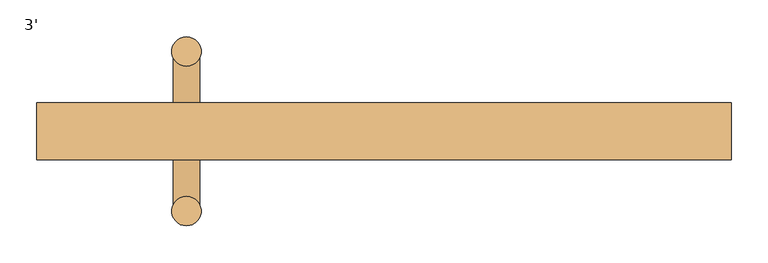
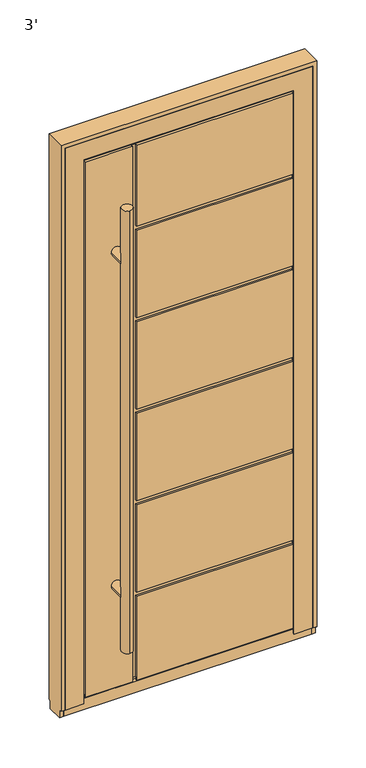
"""IFC4 building model written with IfcOpenShell, lengths in millimetres: door geometry, 3'."""

from ifc_helpers import new_model, si_unit, point, frame, frame_2d, origin, place, context, project, spatial, circle_curve, trimmed, segment, composite_curve, outline, extrude, faceted_brep, source, transform, mapped, element, save


def door_3_5c4206ef(model_context):
    return source(origin(), model_context, "Body", "SolidModel", [
        extrude(outline(composite_curve([segment(trimmed(circle_curve(frame_2d((-268.65, -90.8003001)), 20.0), [point((-268.65, -70.8003001))], [point((-268.65, -110.8003001))], False, "CARTESIAN"), True, "CONTINUOUS"), segment(trimmed(circle_curve(frame_2d((-268.65, -90.8003001)), 20.0), [point((-268.65, -110.8003001))], [point((-268.65, -70.8003001))], False, "CARTESIAN"), True, "CONTINUOUS")], self_intersect=False)), frame((0.0, 0.0, 210.0000003), z_axis=(0.0, 0.0, 1.0), x_axis=(1.0, 0.0, 0.0)), (0.0, 0.0, 1.0), 1724.5),
        extrude(outline(composite_curve([segment(trimmed(circle_curve(frame_2d((-268.65, 126.2003001)), 20.0), [point((-268.65, 146.2003001))], [point((-268.65, 106.2003001))], False, "CARTESIAN"), True, "CONTINUOUS"), segment(trimmed(circle_curve(frame_2d((-268.65, 126.2003001)), 20.0), [point((-268.65, 106.2003001))], [point((-268.65, 146.2003001))], False, "CARTESIAN"), True, "CONTINUOUS")], self_intersect=False)), frame((0.0, 0.0, 210.0000003), z_axis=(0.0, 0.0, 1.0), x_axis=(1.0, 0.0, 0.0)), (0.0, 0.0, 1.0), 1724.5),
        extrude(outline(composite_curve([segment(trimmed(circle_curve(frame_2d((422.2500003, -268.65)), 18.0), [point((422.2500003, -286.65))], [point((422.2500003, -250.65))], False, "CARTESIAN"), True, "CONTINUOUS"), segment(trimmed(circle_curve(frame_2d((422.2500003, -268.65)), 18.0), [point((422.2500003, -250.65))], [point((422.2500003, -286.65))], False, "CARTESIAN"), True, "CONTINUOUS")], self_intersect=False)), frame((0.0, -90.8, 0.0), z_axis=(0.0, 1.0, 0.0), x_axis=(0.0, 0.0, 1.0)), (0.0, 0.0, 1.0), 217.0),
        extrude(outline(composite_curve([segment(trimmed(circle_curve(frame_2d((1722.2500003, -268.65)), 18.0), [point((1722.2500003, -286.65))], [point((1722.2500003, -250.65))], False, "CARTESIAN"), True, "CONTINUOUS"), segment(trimmed(circle_curve(frame_2d((1722.2500003, -268.65)), 18.0), [point((1722.2500003, -250.65))], [point((1722.2500003, -286.65))], False, "CARTESIAN"), True, "CONTINUOUS")], self_intersect=False)), frame((0.0, -90.8, 0.0), z_axis=(0.0, 1.0, 0.0), x_axis=(0.0, 0.0, 1.0)), (0.0, 0.0, 1.0), 217.0),
        faceted_brep([(-193.65, -13.8, 366.5833337), (-193.65, -13.8, 708.166667), (383.65, -13.8, 708.166667), (383.65, -13.8, 723.166667), (-193.65, -13.8, 723.166667), (-193.65, -13.8, 1064.7500004), (383.65, -13.8, 1064.7500004), (383.65, -13.8, 1079.7500004), (-193.65, -13.8, 1079.7500004), (-193.65, -13.8, 1421.3333337), (383.65, -13.8, 1421.3333337), (383.65, -13.8, 1436.3333337), (-193.65, -13.8, 1436.3333337), (-193.65, -13.8, 1777.916667), (383.65, -13.8, 1777.916667), (383.65, -13.8, 1792.916667), (-193.65, -13.8, 1792.916667), (-193.65, -13.8, 2109.5000003), (-208.65, -13.8, 2109.5000003), (-208.65, -13.8, 35.0), (-193.65, -13.8, 35.0), (-193.65, -13.8, 351.5833337), (383.65, -13.8, 351.5833337), (383.65, -13.8, 366.5833337), (-193.65, -20.8, 366.5833337), (-193.65, -20.8, 708.166667), (383.65, -20.8, 708.166667), (383.65, -11.7997698, 2109.5000003), (383.65, -20.8, 2109.5000003), (383.65, -20.8, 1792.916667), (383.65, -20.8, 1777.916667), (383.65, -20.8, 1436.3333337), (383.65, -20.8, 1421.3333337), (383.65, -20.8, 1079.7500004), (383.65, -20.8, 1064.7500004), (383.65, -20.8, 723.166667), (383.65, -20.8, 366.5833337), (383.65, -20.8, 351.5833337), (383.65, -20.8, 24.0), (383.65, -18.8020472, 24.0), (383.65, -18.8020472, 35.0), (383.65, -11.7997698, 35.0), (-193.65, -20.8, 723.166667), (-193.65, -20.8, 1064.7500004), (-193.65, -20.8, 1079.7500004), (-193.65, -20.8, 1421.3333337), (-208.65, -20.8, 2109.5000003), (-208.65, -20.8, 24.0), (-208.65, -18.8020472, 24.0), (-208.65, -18.8020472, 35.0), (-193.65, -18.8020472, 35.0), (-383.65, -18.8020472, 35.0), (-383.65, -11.7997698, 35.0), (-193.65, -20.8, 351.5833337), (-193.65, -18.8020472, 24.0), (-193.65, -20.8, 24.0), (-383.65, -18.8020472, 24.0), (-383.65, -20.8, 24.0), (-383.65, -20.8, 2109.5000003), (-193.65, -20.8, 1777.916667), (-193.65, -20.8, 1436.3333337), (-193.65, -20.8, 2109.5000003), (-193.65, -20.8, 1792.916667), (408.65, 56.2, 10.0000003), (408.65, 53.2, 10.0000003), (-193.65, 53.2, 10.0000003), (-193.65, 56.2, 10.0000003), (-408.65, 53.2, 10.0000003), (-408.65, 56.2, 10.0000003), (-208.65, 56.2, 10.0000003), (-208.65, 53.2, 10.0000003), (408.65, 56.2, 351.5833337), (408.65, 53.2, 351.5833337), (408.65, 56.2, 366.5833337), (408.65, 56.2, 708.166667), (408.65, 53.2, 708.166667), (408.65, 53.2, 366.5833337), (408.65, 56.2, 1079.7500004), (408.65, 56.2, 1421.3333337), (408.65, 53.2, 1421.3333337), (408.65, 53.2, 1079.7500004), (408.65, 56.2, 723.166667), (408.65, 56.2, 1064.7500004), (408.65, 53.2, 1064.7500004), (408.65, 53.2, 723.166667), (408.65, 56.2, 1436.3333337), (408.65, 56.2, 1777.916667), (408.65, 53.2, 1777.916667), (408.65, 53.2, 1436.3333337), (408.65, 56.2, 2134.5000003), (408.65, 53.2, 2134.5000003), (408.65, 53.2, 1792.916667), (408.65, 56.2, 1792.916667), (393.15, 53.2, 351.5833337), (393.15, 53.2, 25.5), (-193.65, 53.2, 25.5), (393.15, 53.2, 708.166667), (393.15, 53.2, 366.5833337), (393.15, 53.2, 1421.3333337), (393.15, 53.2, 1079.7500004), (393.15, 53.2, 1064.7500004), (393.15, 53.2, 723.166667), (393.15, 53.2, 1777.916667), (393.15, 53.2, 1436.3333337), (-193.65, 53.2, 2134.5000003), (-193.65, 53.2, 2119.0000003), (393.15, 53.2, 2119.0000003), (393.15, 53.2, 1792.916667), (-393.15, 53.2, 25.5), (-393.15, 53.2, 2119.0000003), (-208.65, 53.2, 2119.0000003), (-208.65, 53.2, 2134.5000003), (-408.65, 53.2, 2134.5000003), (-208.65, 53.2, 25.5), (-193.65, 49.2, 351.5833337), (-193.65, 56.2, 351.5833337), (-193.65, 49.2, 25.5), (-193.65, 56.2, 366.5833337), (-193.65, 56.2, 708.166667), (-193.65, 56.2, 1079.7500004), (-193.65, 56.2, 1421.3333337), (-193.65, 56.2, 723.166667), (-193.65, 56.2, 1064.7500004), (-193.65, 56.2, 1436.3333337), (-193.65, 56.2, 1777.916667), (-193.65, 56.2, 1792.916667), (-193.65, 56.2, 2134.5000003), (-408.65, 56.2, 2134.5000003), (-208.65, 56.2, 2134.5000003), (-208.65, 49.2, 2119.0000003), (-208.65, 49.2, 25.5), (-383.65, -11.7997698, 2109.5000003), (393.15, -11.7997698, 2119.0000003), (-393.15, -11.7997698, 2119.0000003), (-393.15, -11.7997698, 25.5), (393.15, -11.7997698, 25.5), (393.15, 49.2, 351.5833337), (393.15, 49.2, 366.5833337), (393.15, 49.2, 708.166667), (393.15, 49.2, 723.166667), (393.15, 49.2, 1064.7500004), (393.15, 49.2, 1079.7500004), (393.15, 49.2, 1421.3333337), (393.15, 49.2, 1436.3333337), (393.15, 49.2, 1777.916667), (393.15, 49.2, 1792.916667), (-193.65, 49.2, 1777.916667), (-193.65, 49.2, 1436.3333337), (-193.65, 49.2, 1421.3333337), (-193.65, 49.2, 1079.7500004), (-193.65, 49.2, 1064.7500004), (-193.65, 49.2, 723.166667), (-193.65, 49.2, 708.166667), (-193.65, 49.2, 366.5833337), (-193.65, 49.2, 2119.0000003), (-193.65, 49.2, 1792.916667)], [[[0, 1, 2, 3, 4, 5, 6, 7, 8, 9, 10, 11, 12, 13, 14, 15, 16, 17, 18, 19, 20, 21, 22, 23]], [[1, 0, 24, 25]], [[1, 25, 26, 2]], [[27, 28, 29, 15, 14, 30, 31, 11, 10, 32, 33, 7, 6, 34, 35, 3, 2, 26, 36, 23, 22, 37, 38, 39, 40, 41]], [[42, 4, 3, 35]], [[5, 4, 42, 43]], [[5, 43, 34, 6]], [[44, 8, 7, 33]], [[9, 8, 44, 45]], [[19, 18, 46, 47, 48, 49]], [[41, 40, 50, 20, 19, 49, 51, 52]], [[53, 21, 20, 50, 54, 55]], [[21, 53, 37, 22]], [[24, 0, 23, 36]], [[40, 39, 54, 50]], [[56, 51, 49, 48]], [[39, 38, 55, 54]], [[57, 56, 48, 47]], [[33, 32, 45, 44]], [[35, 34, 43, 42]], [[36, 26, 25, 24]], [[55, 38, 37, 53]], [[58, 57, 47, 46]], [[31, 30, 59, 60]], [[28, 61, 62, 29]], [[63, 64, 65, 66]], [[67, 68, 69, 70]], [[64, 63, 71, 72]], [[73, 74, 75, 76]], [[77, 78, 79, 80]], [[81, 82, 83, 84]], [[85, 86, 87, 88]], [[89, 90, 91, 92]], [[65, 64, 72, 93, 94, 95]], [[76, 75, 96, 97]], [[80, 79, 98, 99]], [[84, 83, 100, 101]], [[88, 87, 102, 103]], [[90, 104, 105, 106, 107, 91]], [[108, 109, 110, 111, 112, 67, 70, 113]], [[114, 115, 66, 65, 95, 116]], [[63, 66, 115, 71]], [[74, 73, 117, 118]], [[78, 77, 119, 120]], [[82, 81, 121, 122]], [[86, 85, 123, 124]], [[89, 92, 125, 126]], [[68, 127, 128, 69]], [[68, 67, 112, 127]], [[129, 130, 113, 70, 69, 128, 111, 110]], [[58, 131, 52, 51, 56, 57]], [[132, 133, 134, 135], [131, 27, 41, 52]], [[106, 132, 135, 94, 93, 136, 137, 97, 96, 138, 139, 101, 100, 140, 141, 99, 98, 142, 143, 103, 102, 144, 145, 107]], [[94, 135, 134, 108, 113, 130, 116, 95]], [[133, 109, 108, 134]], [[146, 147, 143, 142, 148, 149, 141, 140, 150, 151, 139, 138, 152, 153, 137, 136, 114, 116, 130, 129, 154, 155, 145, 144]], [[149, 148, 120, 119]], [[149, 119, 77, 80, 99, 141]], [[122, 150, 140, 100, 83, 82]], [[151, 150, 122, 121]], [[151, 121, 81, 84, 101, 139]], [[118, 152, 138, 96, 75, 74]], [[153, 152, 118, 117]], [[153, 117, 73, 76, 97, 137]], [[115, 114, 136, 93, 72, 71]], [[9, 45, 32, 10]], [[60, 12, 11, 31]], [[13, 12, 60, 59]], [[13, 59, 30, 14]], [[62, 16, 15, 29]], [[16, 62, 61, 17]], [[124, 146, 144, 102, 87, 86]], [[125, 155, 154, 105, 104, 126]], [[120, 148, 142, 98, 79, 78]], [[147, 123, 85, 88, 103, 143]], [[147, 146, 124, 123]], [[155, 125, 92, 91, 107, 145]], [[90, 89, 126, 104]], [[127, 112, 111, 128]], [[132, 106, 105, 154, 129, 110, 109, 133]], [[27, 131, 58, 46, 18, 17, 61, 28]]]),
        faceted_brep([(-457.2, 56.2, 0.0), (-412.7, 56.2, 0.0), (-412.7, 47.2, 0.0), (-457.2, 47.1997571, 0.0), (-403.2, -16.2999958, 0.0), (-387.7, -16.2999958, 0.0), (-387.7, -20.8, 0.0), (-457.2, -20.8, 0.0), (-457.2, -11.8, 0.0), (-403.2, -11.8, 0.0), (457.2, -20.8, 0.0), (387.7, -20.8, 0.0), (387.7, -16.2999958, 0.0), (403.2, -16.2999958, 0.0), (403.2, -11.8, 0.0), (457.2, -11.8, 0.0), (412.7, 47.2, 0.0), (412.7, 56.2, 0.0), (457.2, 56.2, 0.0), (457.2, 47.1997571, 0.0), (-457.2, -20.8, 2189.5), (-457.2, 56.2, 2189.5), (-457.2, 47.1997571, -30.0), (-457.2, -11.8, -30.0), (457.2, 56.2, 2189.5), (412.7, 56.2, 2145.0), (-412.7, 56.2, 2145.0), (457.2, -20.8, 2189.5), (457.2, -11.8, -30.0), (457.2, 47.1997571, -30.0), (-387.7, -20.8, 2120.0), (387.7, -20.8, 2120.0), (-403.2, 47.2, 2135.5), (-403.2, -16.2999958, 2135.5), (-403.2, -11.8, 14.5), (-403.2, 47.2, 14.5), (403.2, 47.2, 2135.5), (403.2, -16.2999958, 2135.5), (403.2, 47.2, 14.5), (403.2, -11.8, 14.5), (-412.7, 47.2, 2145.0), (412.7, 47.2, 2145.0), (387.7, -16.2999958, 2120.0), (-387.7, -16.2999958, 2120.0)], [[[0, 1, 2, 3]], [[4, 5, 6, 7, 8, 9]], [[10, 11, 12, 13, 14, 15]], [[16, 17, 18, 19]], [[7, 20, 21, 0, 3, 22, 23, 8]], [[1, 0, 21, 24, 18, 17, 25, 26]], [[21, 20, 27, 24]], [[18, 24, 27, 10, 15, 28, 29, 19]], [[7, 6, 30, 31, 11, 10, 27, 20]], [[32, 33, 4, 9, 34, 35]], [[33, 32, 36, 37]], [[37, 36, 38, 39, 14, 13]], [[40, 2, 1, 26]], [[16, 19, 29, 22, 3, 2, 40, 41], [36, 32, 35, 38]], [[5, 4, 33, 37, 13, 12, 42, 43]], [[6, 5, 43, 30]], [[26, 25, 41, 40]], [[31, 30, 43, 42]], [[17, 16, 41, 25]], [[12, 11, 31, 42]], [[23, 28, 15, 14, 39, 34, 9, 8]], [[38, 35, 34, 39]], [[23, 22, 29, 28]]]),
        faceted_brep([(-457.2, 47.2, -30.0), (-457.2, -11.8, -30.0), (-472.2, -11.8, -30.0), (-472.2, 47.2, -30.0), (-457.2, 56.2, 2189.5), (-457.2, -20.8, 2189.5), (-457.2, -20.8, 0.0), (-457.2, -11.8, 0.0), (-457.2, 47.2, 0.0), (-457.2, 56.2, 0.0), (472.2, -11.8, 0.0), (457.2, -11.8, 0.0), (457.2, -11.8, -30.0), (472.2, -11.8, -30.0), (-472.2, -11.8, 0.0), (-472.2, -20.8, 2204.5), (-472.2, 56.2, 2204.5), (-472.2, 56.2, 0.0), (-472.2, 47.2, 0.0), (-472.2, -20.8, 0.0), (457.2, 47.2, 0.0), (472.2, 47.2, 0.0), (472.2, 47.2, -30.0), (457.2, 47.2, -30.0), (457.2, -20.8, 2189.5), (457.2, 56.2, 2189.5), (457.2, 56.2, 0.0), (457.2, -20.8, 0.0), (472.2, 56.2, 2204.5), (472.2, 56.2, 0.0), (472.2, -20.8, 0.0), (472.2, -20.8, 2204.5)], [[[0, 1, 2, 3]], [[4, 5, 6, 7, 1, 0, 8, 9]], [[10, 11, 12, 13]], [[7, 14, 2, 1]], [[15, 16, 17, 18, 3, 2, 14, 19]], [[20, 21, 22, 23]], [[18, 8, 0, 3]], [[24, 25, 26, 20, 23, 12, 11, 27]], [[25, 4, 9, 17, 16, 28, 29, 26]], [[21, 20, 26, 29]], [[8, 18, 17, 9]], [[22, 13, 12, 23]], [[11, 10, 30, 27]], [[14, 7, 6, 19]], [[5, 24, 27, 30, 31, 15, 19, 6]], [[28, 31, 30, 10, 13, 22, 21, 29]], [[5, 4, 25, 24]], [[16, 15, 31, 28]]]),
    ])


if __name__ == "__main__":
    model = new_model("IFC4")
    model_context = context("Model", 3, world=origin())
    ifc_project = project(units=[si_unit("LENGTHUNIT", "METRE", prefix="MILLI")], contexts=[model_context])
    site = spatial("IfcSite", under=ifc_project)
    building = spatial("IfcBuilding", under=site)
    placement = place(None, origin())
    door_3_shape = door_3_5c4206ef(model_context)
    element("IfcDoor", 1, ObjectType="3'", at=placement, inside=building, context=model_context, shape_type="MappedRepresentation", body=[
        mapped(door_3_shape, transform((0.0, 0.0, 0.0), x_axis=(1.0, 0.0, 0.0), y_axis=(0.0, 1.0, 0.0), z_axis=(0.0, 0.0, 1.0))),
    ])
    save(model, "model.ifc")

# Revit data of these elements
# Type "3'"
#   Type Mark = "10"
#   Water resistance = "up to Class E900, EN 12208:2001"
#   Uniclass2015Version = "v1.21"
#   Uniclass2015Reference = "Ss_25_30_20_30"
#   Uniclass2015Description = "Frame and door leaf system"
#   URL = "www.aluprof.com"
#   Type IFC Predefined Type = "USERDEFINED"
#   Right-hand / Left-hand door [instance default] = ""
#   Resistance to wind load = "up to Class C5/B5, EN 12210:2001"
#   Insert type = "ST"
#   Hardware [instance default] = ""
#   Product page = "https://aluprof.com/en/architects/offer/window-and-door-systems/panel-doors#visualisation"
#   Operation = "SinglePanelOutwardOpening"
#   Opening type = "Outward"
#   NBSReference = "25-50-20/125"
#   NBSDescription = "Frame and door leaf system"
#   Important = "The actual acceptable construction dimensions are dependent on the selection of profiles and hardware, glazing type, construction weight and the construction’s operating conditions. These should be determined by a suitably qualified person, and using ALUPROF’s calculation software"
#   IfcExportType = "USERDEFINED"
#   IfcExportAs = "IfcDoorType"
#   Handle type [instance default] = ""
#   Manufacturer = "ALUPROF SA"
#   Export Type to IFC As = "IfcDoorType"
#   Door sill type [instance default] = ""
#   Description = "External single-leaf panel door outward opening"
#   Model = "MB-86 ST Panel Door AD07"
#   Content of the recyclate in the material = "69.2%"
#   COBie.Type.WarrantyDurationParts = ""
#   COBie.Type.Name = ""
#   COBie.Type.Manufacturer = "ALUPROF SA"
#   COBie.Space.Name = ""
#   COBie.Floor.Name = ""
#   COBie.Facility.Name = ""
#   COBie.CreatedOn = ""
#   COBie.Component.WarrantyStartDate = ""
#   COBie.Component.Name = "MB-86 ST Panel Door AD07"
#   Burglar resistance = "RC2"
#   Air permeability = "up to Class 4, EN 12207:2001"
#   Width of the active leaf = 2' - 8.17717"
#   Placement in wall = 0' - 0.7874"
#   Thickness = 0' - 3.0315"
#   Height of the opening sash = 6' - 11.64173"
#   Handle Offset = 3' - 5.33858"
#   Rough Height = 7' - 4.61024"
#   Rough Width = 3' - 1.1811"
#   Height = 7' - 2.20079"
#   Width = 3' - 0"
#   Construction depth = 0' - 3.0315"
#   Clear opening width = 2' - 3.94882"
#   Clear opening height = 6' - 10.67717"
#   Height of the array = 1' - 1.44816"
#   Schedule No. [instance default] = 1
#   Handrail [instance default] = yes
#   IsExternal = yes
#   Handle [instance default] = no
#   Door closer [instance default] = no
#   Function = 1
#   COBie.Type = yes
#   COBie = yes
#   Access control [instance default] = no
#   Panel = element 346771
#   Wall Closure = (empty or 0)
